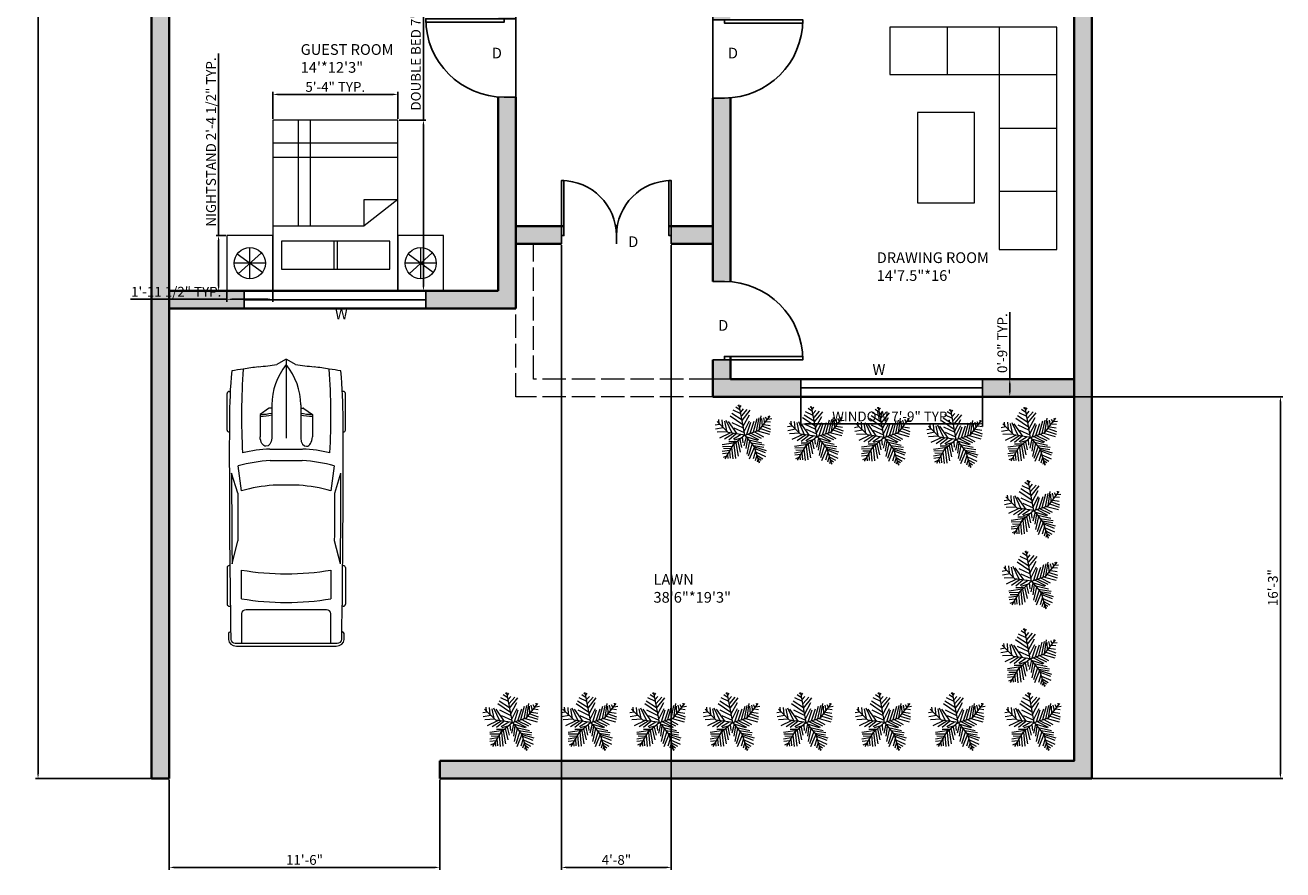
# Model space of a CAD drawing. Units: inches. Extents: x 1658 to 2301, y 1028 to 1972.
# Tile 1 of 2: x 1658 to 2301, y 1028 to 1460. Entities that reach past the tile are written whole.
import ezdxf

# ---------------------------------------------------------------- set-up
doc = ezdxf.new("R2010")
doc.units = ezdxf.units.IN
doc.linetypes.add('ACAD_ISO02W100', pattern=[15, 12, -3])
for name, color, linetype, lineweight in [('A-ANNO-DIMS', 31, 'Continuous', 18), ('A-AREA-IDEN', 31, 'Continuous', 18), ('A-WALL-OVHD', 140, 'ACAD_ISO02W100', 18), ('A-WALL-PATT', 140, 'Continuous', 13), ('DOOR', 54, 'Continuous', 25), ('FUR', 181, 'Continuous', 18), ('L-SITE-VEHI', 8, 'Continuous', 18), ('L-SITE-WALL', 140, 'Continuous', 35), ('TEXT', 31, 'Continuous', 18), ('TREE', 90, 'Continuous', 13), ('WALL', 140, 'Continuous', 35), ('WIND', 211, 'Continuous', 25)]:
    doc.layers.add(name, color=color, linetype=linetype, lineweight=lineweight)
doc.styles.get("Standard").update_dxf_attribs({"font": 'arial.ttf'})
doc.dimstyles.new('ISO-25', dxfattribs={"dimtxt": 5, "dimasz": 2.5, "dimexe": 1.25, "dimexo": 0.625, "dimtad": 1, "dimdec": 0, "dimlunit": 4, "dimtxsty": 'Standard', "dimcen": 2.5, "dimadec": 0, "dimazin": 0, "dimtfac": 1, "dimtdec": 0, "dimtmove": 0, "dimatfit": 3, "dimfxl": 1, "dimarcsym": 0})

# ---------------------------------------------------------------- blocks, each defined once
blk = doc.blocks.new('*U6')
for p, q in [((21.1, 37.41), (21.1, 36.83)), ((46.55, 38.89), (22.35, 38.89)), ((47.8, 37.39), (47.8, 37.41)), ((87.99, 31.87), (74.76, 35.92)), ((134.31, 35.6), (119.29, 31.78)), ((135.45, 37.07), (135.45, 37.41)), ((136.7, 38.89), (160.9, 38.89)), ((162.15, 37.41), (162.15, 36.77)), ((186.47, -33.5), (186.47, 33.5)), ((70.03, 31.54), (86.41, 29.35)), ((138.42, 29.35), (157.25, 29.35)), ((164.52, 26.39), (164.52, -26.39)), ((186.47, 29.35), (167.01, 29.35)), ((188.4, -32.76), (188.4, 32.76)), ((32.27, 11.63), (36.13, 17.17)), ((36.13, 17.17), (50.94, 17.17)), ((29.77, 9.51), (51.68, 9.51)), ((32.12, 9.51), (32.12, 11.15)), ((58.92, -10.77), (58.92, 10.77)), ((66.55, -10.53), (66.55, 10.53)), ((82.74, 8.5), (82.74, -8.5)), ((186.47, -10.53), (186.47, 10.53)), ((3.27, 6.13), (0.1, 0.41)), ((0, 0), (51.68, 0)), ((0.1, -0.41), (3.27, -6.13)), ((29.77, -9.51), (51.68, -9.51)), ((32.12, -9.51), (32.12, -11.15)), ((32.27, -11.63), (36.13, -17.17)), ((36.13, -17.17), (50.94, -17.17)), ((86.41, -29.35), (70.03, -31.54)), ((87.99, -31.87), (74.76, -35.92)), ((134.31, -35.6), (119.29, -31.78)), ((157.25, -29.35), (138.42, -29.35)), ((167.01, -29.35), (186.47, -29.35)), ((21.1, -37.41), (21.1, -36.83)), ((46.55, -38.89), (22.35, -38.89)), ((47.8, -37.39), (47.8, -37.41)), ((135.45, -37.07), (135.45, -37.41)), ((136.7, -38.89), (160.9, -38.89)), ((162.15, -37.41), (162.15, -36.77))]:
    blk.add_line(p, q)
for centre, major_axis, ratio, start_param, end_param in [((266.03, -27.52), (0, 313.31), 0.842304, 1.367076, 1.39176), ((41.19, -490.86), (0, 528.23), 0.842304, 0.00281, 0.075598), ((22.35, 37.41), (0, -1.48), 0.842304, 3.141593, 4.712389), ((64.48, -10555.62), (0, 10593.03), 0.842304, -0.013397, 0.002797), ((46.55, 37.41), (0, 1.48), 0.842304, -1.570796, 0), ((64.48, -10555.62), (0, -10591.55), 0.842304, 3.133765, 3.140441), ((136.7, 37.41), (0, -1.48), 0.842304, 3.141593, 4.712389), ((160.9, 37.41), (0, 1.48), 0.842304, -1.570796, 0), ((180.63, 35.84), (0, 2.22), 0.842304, -0.013017, 1.249894), ((64.48, -10556.36), (0, 10595.31), 0.842304, -0.013397, -0.013017), ((183.98, 33.5), (0, -2.96), 0.842304, 1.570796, 3.128196), ((183.98, 32.76), (0, -5.25), 0.842304, 1.570796, 3.128196), ((259.18, -27.52), (0, -305.3), 0.842304, 4.528606, 4.561838), ((37.47, -593.96), (0, -623.33), 0.842304, 3.096046, 3.200911), ((134.4, 5.39), (0, -89.78), 0.842304, 4.449482, 4.652344), ((135.29, 5.39), (0, 81.77), 0.842304, 1.245306, 1.50788), ((149.6, 2.8), (0, -79.58), 0.842304, 4.372215, 4.640744), ((95.79, -3666.35), (0, -3698.24), 0.842304, 3.134049, 3.144098), ((17.08, 0), (0, 147.02), 0.842304, 4.511394, 4.913384), ((35.91, 0), (0, 147.02), 0.842304, 4.511394, 4.913384), ((167.01, 26.39), (0, 2.96), 0.842304, 0, 1.570796), ((-204.49, 52.4), (0, -250.96), 0.842304, 1.385369, 1.434372), ((13.04, 17.01), (0, 27.42), 0.842304, 4.435146, 4.718221), ((14.2, 17.01), (0, 27.42), 0.842304, 4.435146, 4.718221), ((50.79, 13.34), (6.34, -0.36), 0.603834, -1.395552, 1.581315), ((29.77, -46.66), (0, 56.17), 0.842304, 0, 0.590319), ((32.75, 11.15), (0, 0.74), 0.842304, 0.879714, 1.570796), ((0.62, 0), (0, -0.74), 0.842304, 4.131459, 5.293319), ((-204.49, -52.4), (0, 250.96), 0.842304, -1.434372, -1.385369), ((29.77, 46.66), (0, 56.17), 0.842304, 2.551274, 3.141593), ((32.75, -11.15), (0, -0.74), 0.842304, 4.712389, 5.403472), ((13.04, -17.01), (0, -27.42), 0.842304, 1.564964, 1.848039), ((14.2, -17.01), (0, -27.42), 0.842304, 1.564964, 1.848039), ((134.4, -5.39), (0, -89.78), 0.842304, -1.510751, -1.307889), ((135.29, -5.39), (0, -81.77), 0.842304, -1.50788, -1.245306), ((149.6, -2.8), (0, -79.58), 0.842304, -1.499151, -1.230623), ((259.18, 27.52), (0, 305.3), 0.842304, 1.721348, 1.754579), ((266.03, 27.52), (0, 313.31), 0.842304, 1.749832, 1.774517), ((37.47, 593.96), (0, -623.33), 0.842304, -0.059319, 0.045547), ((95.79, 3666.35), (0, -3698.24), 0.842304, -0.002505, 0.007544), ((167.01, -26.39), (0, -2.96), 0.842304, 4.712389, 6.283185), ((183.98, -32.76), (0, -5.25), 0.842304, 0.013397, 1.570796), ((41.19, 490.86), (0, -528.23), 0.842304, -0.075598, -0.00281), ((22.35, -37.41), (0, 1.48), 0.842304, 1.570796, 3.141593), ((64.48, 10555.62), (0, 10593.03), 0.842304, 3.138796, 3.15499), ((46.55, -37.41), (0, -1.48), 0.842304, 0, 1.570796), ((64.48, 10555.62), (0, -10591.55), 0.842304, 0.001152, 0.007828), ((136.7, -37.41), (0, -1.48), 0.842304, -1.570796, 0), ((160.9, -37.41), (0, 1.48), 0.842304, 3.141593, 4.712389), ((180.63, -35.84), (0, -2.22), 0.842304, -1.249894, 0.013017), ((64.48, 10556.36), (0, 10595.31), 0.842304, 3.15461, 3.15499), ((183.98, -33.5), (0, 2.96), 0.842304, 3.15499, 4.712389)]:
    blk.add_ellipse(centre, major_axis=major_axis, ratio=ratio, start_param=start_param, end_param=end_param)
at = {"extrusion": (0, 0, -1)}
blk.add_ellipse((50.79, -13.34), major_axis=(6.34, 0.36), ratio=0.603834, start_param=-1.395552, end_param=1.581315, dxfattribs=at)
blk = doc.blocks.new('*U2')
for p, q in [((0, 0), (0, -6)), ((40, 0), (40, -6))]:
    blk.add_line(p, q)
blk.add_lwpolyline([(0, 0), (0, 40), (1.75, 40), (1.75, 0)], close=True)
blk.add_arc((0, 0), 40, 0, 90)
blk = doc.blocks.new('*U8')
for p, q in [((-8.737, 47.138), (-17.069, 52.711)), ((-10.186, 53.64), (-13.084, 55.962)), ((0, 0), (-10.5, 57)), ((-9.099, 51.782), (-6.563, 55.962)), ((-7.65, 43.423), (-2.578, 49.46)), ((-5.839, 35.992), (4.667, 48.067)), ((-31.5, 4.5), (-52.5, 25.5)), ((-48.585, 21.131), (-49.309, 29.026)), ((-43.513, 28.561), (-42.427, 15.558)), ((-38.442, 26.239), (-34.819, 7.663)), ((-35.544, 28.097), (-24.314, 3.947)), ((-14.533, 2.09), (-30.834, 25.31)), ((-3.665, 19.273), (-27.574, 35.527)), ((-5.114, 28.097), (-24.676, 40.636)), ((-24.314, 23.917), (-2.941, 13.7)), ((-7.288, 39.707), (-21.778, 46.673)), ((-5.114, 27.632), (10.463, 46.673)), ((-2.941, 16.486), (8.652, 37.85)), ((-1.129, 6.734), (9.014, 26.704)), ((3.942, 1.625), (11.187, 24.381)), ((10.101, 3.483), (17.708, 26.239)), ((16.259, 5.805), (23.142, 31.348)), ((22.055, 7.198), (27.489, 32.277)), ((27, 9), (48, 36)), ((27.127, 9.056), (31.112, 35.992)), ((31.836, 30.883), (32.561, 16.486)), ((35.096, 32.741), (37.27, 22.524)), ((38.719, 34.134), (41.979, 28.561)), ((40.53, 25.775), (48.862, 24.846)), ((43.791, 29.954), (51.036, 30.883)), ((44.153, 36.456), (45.239, 32.741)), ((-47.498, 19.737), (-55.83, 18.344)), ((-40.615, 13.7), (-55.105, 10.913)), ((-33.37, 6.269), (-52.207, 5.34)), ((-28.299, 3.483), (-47.86, -5.805)), ((-21.416, 3.018), (-38.079, -8.128)), ((0, 0), (-31.5, 4.5)), ((-15.982, 2.09), (-30.11, -9.521)), ((0, 0), (-22.5, -19.5)), ((-6.563, 1.161), (-21.416, -8.128)), ((-20.691, 13.7), (-1.129, 4.876)), ((0, 0), (27, 9)), ((0, 0), (18, -22.5)), ((6.478, 1.625), (26.04, -8.592)), ((11.187, 3.483), (30.749, -5.805)), ((18.07, 5.805), (35.096, -3.483)), ((24.229, 7.663), (46.688, 1.625)), ((29.662, 12.307), (48.137, 6.269)), ((33.285, 16.486), (48.862, 10.913)), ((36.183, 19.737), (48.137, 17.88)), ((-17.431, -15.094), (-42.789, -18.809)), ((-24.314, -21.596), (-42.427, -22.06)), ((-22.5, -19.5), (-37.5, -45)), ((-15.257, -12.772), (-30.11, -12.772)), ((-20.691, -18.345), (-17.793, -44.352)), ((-6.563, -5.805), (-19.967, -9.985)), ((-17.069, -15.094), (-12.721, -40.172)), ((-13.446, -11.378), (-8.737, -32.741)), ((-9.461, -8.592), (-6.201, -23.453)), ((-4.752, -3.483), (-3.665, -14.629)), ((2.493, -3.019), (-1.491, -20.202)), ((1.769, -2.555), (24.229, -9.521)), ((5.029, -6.27), (2.131, -25.775)), ((9.014, -11.378), (3.58, -35.992)), ((14.085, -16.951), (6.478, -40.172)), ((7.565, -9.056), (32.198, -14.629)), ((18.07, -22.524), (8.289, -45.745)), ((12.274, -15.094), (36.907, -18.809)), ((16.259, -19.738), (36.183, -22.989)), ((18, -22.5), (27, -52.5)), ((18.433, -22.524), (40.53, -29.026)), ((-28.299, -29.026), (-42.789, -31.348)), ((-30.834, -34.135), (-42.427, -35.528)), ((-34.457, -39.708), (-40.978, -42.494)), ((-26.849, -26.24), (-40.253, -25.775)), ((-32.646, -36.921), (-31.921, -44.352)), ((-29.023, -30.884), (-27.936, -43.887)), ((-25.038, -23.918), (-22.865, -45.281)), ((20.244, -30.419), (15.897, -44.816)), ((19.157, -25.311), (38.719, -33.206)), ((22.78, -37.85), (19.519, -48.532)), ((21.331, -32.741), (39.081, -40.636)), ((22.78, -38.314), (34.372, -44.816)), ((24.591, -45.745), (23.142, -50.854)), ((24.591, -43.423), (30.749, -47.603)), ((26.764, -49.925), (28.213, -50.854))]:
    blk.add_line(p, q)
blk = doc.blocks.new('*D10')
at = {"layer": 'A-ANNO-DIMS', "color": 0, "lineweight": -2, "transparency": 16777216}
for p, q in [((1722.37, 1915.04), (1663.75, 1915.04)), ((1665, 1912.54), (1665, 1077.54)), ((1722.37, 1075.04), (1663.75, 1075.04))]:
    blk.add_line(p, q, dxfattribs=at)
at = {"layer": 'A-ANNO-DIMS', "color": 0, "lineweight": 100, "transparency": 16777216}
for points in [[(1664.59, 1912.54), (1665.42, 1912.54), (1665, 1915.04)], [(1664.59, 1077.54), (1665.42, 1077.54), (1665, 1075.04)]]:
    blk.add_solid(points, dxfattribs=at)
at = {"layer": 'Defpoints', "color": 0, "lineweight": 100, "transparency": 16777216}
for p in [(1722.99, 1915.04), (1665, 1075.04), (1722.99, 1075.04)]:
    blk.add_point(p, dxfattribs=at)
at = {"layer": 'A-ANNO-DIMS', "color": 0, "transparency": 16777216, "insert": (1661.82, 1495.04), "char_height": 5, "attachment_point": 5, "rotation": 90}
blk.add_mtext("70'", dxfattribs=at)
blk = doc.blocks.new('BED-DOUBLE')
for p, q in [((33.2, 63.87), (33.2, 17.24)), ((68.25, 63.87), (68.25, 0)), ((75.56, 63.87), (75.56, 0)), ((33.2, 50.75), (87.28, 50.75)), ((33.2, 44.52), (87.28, 44.52)), ((33.2, 17.24), (46.75, 17.24)), ((46.75, 0), (33.2, 17.24)), ((46.75, 17.24), (46.75, 0))]:
    blk.add_line(p, q)
for points in [[(0, 0), (87.28, 0), (87.28, 63.87), (0, 63.87)], [(11.05, 30.77), (25.46, 30.77), (25.46, 59.34), (11.05, 59.34)], [(11.05, 4.13), (25.46, 4.13), (25.46, 32.7), (11.05, 32.7)]]:
    blk.add_lwpolyline(points, close=True)
blk = doc.blocks.new('NIGHTSTAND-LAMP')
for p, q in [((14.17, 3.75), (14.17, 19.65)), ((19.52, 5.82), (8.81, 17.58)), ((9.46, 5.29), (18.87, 18.1)), ((6.22, 11.7), (22.11, 11.7))]:
    blk.add_line(p, q)
blk.add_lwpolyline([(0, 0), (28.33, 0), (28.33, 23.39), (0, 23.39)], close=True)
blk.add_circle((14.17, 11.7), 7.95)
blk = doc.blocks.new('WIN-93')
blk.add_line((0, 4.5), (92.82, 4.5))
blk.add_lwpolyline([(0, 0), (92.82, 0), (92.82, 9), (0, 9)], close=True)
blk = doc.blocks.new('*D17')
at = {"layer": 'A-ANNO-DIMS', "color": 0, "lineweight": -2, "transparency": 16777216}
for p, q in [((1861.79, 1411.32), (1861.79, 1503.92)), ((1849.32, 1411.32), (1863.04, 1411.32)), ((1861.79, 1326.54), (1861.79, 1408.82)), ((1849.32, 1324.04), (1863.04, 1324.04))]:
    blk.add_line(p, q, dxfattribs=at)
at = {"layer": 'A-ANNO-DIMS', "color": 0, "lineweight": 100, "transparency": 16777216}
for points in [[(1861.37, 1408.82), (1862.2, 1408.82), (1861.79, 1411.32)], [(1861.37, 1326.54), (1862.2, 1326.54), (1861.79, 1324.04)]]:
    blk.add_solid(points, dxfattribs=at)
at = {"layer": 'Defpoints', "color": 0, "lineweight": 100, "transparency": 16777216}
for p in [(1848.69, 1411.32), (1861.79, 1411.32), (1848.69, 1324.04)]:
    blk.add_point(p, dxfattribs=at)
at = {"layer": 'A-ANNO-DIMS', "color": 0, "transparency": 16777216, "insert": (1858.57, 1458.87), "char_height": 5, "attachment_point": 5, "rotation": 90}
blk.add_mtext('DOUBLE BED 7\'-3 1/2" TYP.', dxfattribs=at)
blk = doc.blocks.new('*D18')
at = {"layer": 'A-ANNO-DIMS', "color": 0, "lineweight": -2, "transparency": 16777216}
for p, q in [((1784.83, 1411.94), (1784.83, 1425.66)), ((1848.69, 1411.94), (1848.69, 1425.66)), ((1846.19, 1424.41), (1787.33, 1424.41))]:
    blk.add_line(p, q, dxfattribs=at)
at = {"layer": 'A-ANNO-DIMS', "color": 0, "lineweight": 100, "transparency": 16777216}
for points in [[(1787.33, 1424.83), (1787.33, 1423.99), (1784.83, 1424.41)], [(1846.19, 1424.83), (1846.19, 1423.99), (1848.69, 1424.41)]]:
    blk.add_solid(points, dxfattribs=at)
at = {"layer": 'Defpoints', "color": 0, "lineweight": 100, "transparency": 16777216}
for p in [(1784.83, 1424.41), (1784.83, 1411.32), (1848.69, 1411.32)]:
    blk.add_point(p, dxfattribs=at)
at = {"layer": 'A-ANNO-DIMS', "color": 0, "transparency": 16777216, "insert": (1816.76, 1427.58), "char_height": 5, "attachment_point": 5}
blk.add_mtext('5\'-4" TYP.', dxfattribs=at)
blk = doc.blocks.new('*D19')
at = {"layer": 'A-ANNO-DIMS', "color": 0, "lineweight": -2, "transparency": 16777216}
for p, q in [((1757.19, 1352.37), (1757.19, 1445.35)), ((1760.81, 1352.37), (1755.94, 1352.37)), ((1757.19, 1326.54), (1757.19, 1349.87)), ((1760.81, 1324.04), (1755.94, 1324.04))]:
    blk.add_line(p, q, dxfattribs=at)
at = {"layer": 'A-ANNO-DIMS', "color": 0, "lineweight": 100, "transparency": 16777216}
for points in [[(1756.77, 1349.87), (1757.6, 1349.87), (1757.19, 1352.37)], [(1756.77, 1326.54), (1757.6, 1326.54), (1757.19, 1324.04)]]:
    blk.add_solid(points, dxfattribs=at)
at = {"layer": 'Defpoints', "color": 0, "lineweight": 100, "transparency": 16777216}
for p in [(1757.19, 1352.37), (1761.43, 1352.37), (1761.43, 1324.04)]:
    blk.add_point(p, dxfattribs=at)
at = {"layer": 'A-ANNO-DIMS', "color": 0, "transparency": 16777216, "insert": (1753.97, 1400.11), "char_height": 5, "attachment_point": 5, "rotation": 90}
blk.add_mtext('NIGHTSTAND 2\'-4 1/2" TYP.', dxfattribs=at)
blk = doc.blocks.new('*D20')
at = {"layer": 'A-ANNO-DIMS', "color": 0, "lineweight": -2, "transparency": 16777216}
for p, q in [((1761.43, 1323.41), (1761.43, 1318.54)), ((1784.83, 1323.41), (1784.83, 1318.54)), ((1761.43, 1319.79), (1712.14, 1319.79)), ((1782.33, 1319.79), (1763.93, 1319.79))]:
    blk.add_line(p, q, dxfattribs=at)
at = {"layer": 'A-ANNO-DIMS', "color": 0, "lineweight": 100, "transparency": 16777216}
for points in [[(1763.93, 1320.21), (1763.93, 1319.37), (1761.43, 1319.79)], [(1782.33, 1320.21), (1782.33, 1319.37), (1784.83, 1319.79)]]:
    blk.add_solid(points, dxfattribs=at)
at = {"layer": 'Defpoints', "color": 0, "lineweight": 100, "transparency": 16777216}
for p in [(1761.43, 1324.04), (1784.83, 1324.04), (1761.43, 1319.79)]:
    blk.add_point(p, dxfattribs=at)
at = {"layer": 'A-ANNO-DIMS', "color": 0, "transparency": 16777216, "insert": (1735.54, 1323), "char_height": 5, "attachment_point": 5}
blk.add_mtext('1\'-11 1/2" TYP.', dxfattribs=at)
blk = doc.blocks.new('*D23')
at = {"layer": 'A-ANNO-DIMS', "color": 0, "lineweight": -2, "transparency": 16777216}
for p, q in [((2054.42, 1269.41), (2054.42, 1254.86)), ((2147.24, 1269.41), (2147.24, 1254.86)), ((2056.92, 1256.11), (2144.74, 1256.11))]:
    blk.add_line(p, q, dxfattribs=at)
at = {"layer": 'A-ANNO-DIMS', "color": 0, "lineweight": 100, "transparency": 16777216}
for points in [[(2056.92, 1256.53), (2056.92, 1255.7), (2054.42, 1256.11)], [(2144.74, 1256.53), (2144.74, 1255.7), (2147.24, 1256.11)]]:
    blk.add_solid(points, dxfattribs=at)
at = {"layer": 'Defpoints', "color": 0, "lineweight": 100, "transparency": 16777216}
for p in [(2054.42, 1270.04), (2147.24, 1270.04), (2147.24, 1256.11)]:
    blk.add_point(p, dxfattribs=at)
at = {"layer": 'A-ANNO-DIMS', "color": 0, "transparency": 16777216, "insert": (2100.83, 1259.33), "char_height": 5, "attachment_point": 5}
blk.add_mtext('WINDOW 7\'-9" TYP.', dxfattribs=at)
blk = doc.blocks.new('*D24')
at = {"layer": 'A-ANNO-DIMS', "color": 0, "lineweight": -2, "transparency": 16777216}
for p, q in [((2161.17, 1279.04), (2161.17, 1313.27)), ((2147.87, 1279.04), (2162.42, 1279.04)), ((2161.17, 1272.54), (2161.17, 1276.54)), ((2147.87, 1270.04), (2162.42, 1270.04))]:
    blk.add_line(p, q, dxfattribs=at)
at = {"layer": 'A-ANNO-DIMS', "color": 0, "lineweight": 100, "transparency": 16777216}
for points in [[(2160.75, 1276.54), (2161.58, 1276.54), (2161.17, 1279.04)], [(2160.75, 1272.54), (2161.58, 1272.54), (2161.17, 1270.04)]]:
    blk.add_solid(points, dxfattribs=at)
at = {"layer": 'Defpoints', "color": 0, "lineweight": 100, "transparency": 16777216}
for p in [(2147.24, 1279.04), (2161.17, 1279.04), (2147.24, 1270.04)]:
    blk.add_point(p, dxfattribs=at)
at = {"layer": 'A-ANNO-DIMS', "color": 0, "transparency": 16777216, "insert": (2157.99, 1297.4), "char_height": 5, "attachment_point": 5, "rotation": 90}
blk.add_mtext('0\'-9" TYP.', dxfattribs=at)
blk = doc.blocks.new('*D29')
at = {"layer": 'A-ANNO-DIMS', "color": 0, "lineweight": -2, "transparency": 16777216}
for p, q in [((2194.62, 1270.04), (2300.59, 1270.04)), ((2299.34, 1267.54), (2299.34, 1077.54)), ((2203.62, 1075.04), (2300.59, 1075.04))]:
    blk.add_line(p, q, dxfattribs=at)
at = {"layer": 'A-ANNO-DIMS', "color": 0, "lineweight": 100, "transparency": 16777216}
for points in [[(2298.92, 1267.54), (2299.76, 1267.54), (2299.34, 1270.04)], [(2298.92, 1077.54), (2299.76, 1077.54), (2299.34, 1075.04)]]:
    blk.add_solid(points, dxfattribs=at)
at = {"layer": 'Defpoints', "color": 0, "lineweight": 100, "transparency": 16777216}
for p in [(2193.99, 1270.04), (2202.99, 1075.04), (2299.34, 1075.04)]:
    blk.add_point(p, dxfattribs=at)
at = {"layer": 'A-ANNO-DIMS', "color": 0, "transparency": 16777216, "insert": (2296.16, 1172.54), "char_height": 5, "attachment_point": 5, "rotation": 90}
blk.add_mtext('16\'-3"', dxfattribs=at)
blk = doc.blocks.new('*D30')
at = {"layer": 'A-ANNO-DIMS', "color": 0, "lineweight": -2, "transparency": 16777216}
for p, q in [((1731.99, 1074.41), (1731.99, 1028.44)), ((1870.11, 1074.41), (1870.11, 1028.44)), ((1734.49, 1029.69), (1867.61, 1029.69))]:
    blk.add_line(p, q, dxfattribs=at)
at = {"layer": 'A-ANNO-DIMS', "color": 0, "lineweight": 100, "transparency": 16777216}
for points in [[(1734.49, 1030.1), (1734.49, 1029.27), (1731.99, 1029.69)], [(1867.61, 1030.1), (1867.61, 1029.27), (1870.11, 1029.69)]]:
    blk.add_solid(points, dxfattribs=at)
at = {"layer": 'Defpoints', "color": 0, "lineweight": 100, "transparency": 16777216}
for p in [(1731.99, 1075.04), (1870.11, 1075.04), (1870.11, 1029.69)]:
    blk.add_point(p, dxfattribs=at)
at = {"layer": 'A-ANNO-DIMS', "color": 0, "transparency": 16777216, "insert": (1801.05, 1032.87), "char_height": 5, "attachment_point": 5}
blk.add_mtext('11\'-6"', dxfattribs=at)
blk = doc.blocks.new('*D31')
at = {"layer": 'A-ANNO-DIMS', "color": 0, "lineweight": -2, "transparency": 16777216}
for p, q in [((1908.99, 1357.76), (1908.99, 1961.64)), ((1911.49, 1960.39), (2006.99, 1960.39)), ((2009.49, 1357.76), (2009.49, 1961.64))]:
    blk.add_line(p, q, dxfattribs=at)
at = {"layer": 'A-ANNO-DIMS', "color": 0, "lineweight": 100, "transparency": 16777216}
for points in [[(1911.49, 1960.8), (1911.49, 1959.97), (1908.99, 1960.39)], [(2006.99, 1960.8), (2006.99, 1959.97), (2009.49, 1960.39)]]:
    blk.add_solid(points, dxfattribs=at)
at = {"layer": 'Defpoints', "color": 0, "lineweight": 100, "transparency": 16777216}
for p in [(2009.49, 1960.39), (1908.99, 1357.13), (2009.49, 1357.13)]:
    blk.add_point(p, dxfattribs=at)
at = {"layer": 'A-ANNO-DIMS', "color": 0, "transparency": 16777216, "insert": (1959.24, 1963.6), "char_height": 5, "attachment_point": 5}
blk.add_mtext('8\'-4 1/2"', dxfattribs=at)
blk = doc.blocks.new('*D32')
at = {"layer": 'A-ANNO-DIMS', "color": 0, "lineweight": -2, "transparency": 16777216}
for p, q in [((1932.24, 1347.51), (1932.24, 1028.44)), ((1988.35, 1347.51), (1988.35, 1028.44)), ((1934.74, 1029.69), (1985.85, 1029.69))]:
    blk.add_line(p, q, dxfattribs=at)
at = {"layer": 'A-ANNO-DIMS', "color": 0, "lineweight": 100, "transparency": 16777216}
for points in [[(1934.74, 1030.1), (1934.74, 1029.27), (1932.24, 1029.69)], [(1985.85, 1030.1), (1985.85, 1029.27), (1988.35, 1029.69)]]:
    blk.add_solid(points, dxfattribs=at)
at = {"layer": 'Defpoints', "color": 0, "lineweight": 100, "transparency": 16777216}
for p in [(1932.24, 1348.13), (1988.35, 1348.13), (1988.35, 1029.69)]:
    blk.add_point(p, dxfattribs=at)
at = {"layer": 'A-ANNO-DIMS', "color": 0, "transparency": 16777216, "insert": (1960.3, 1032.87), "char_height": 5, "attachment_point": 5}
blk.add_mtext('4\'-8"', dxfattribs=at)

msp = doc.modelspace()

# ---------------------------------------------------------------- hatches: boundary and pattern name
at = {"layer": 'A-WALL-PATT'}
h = msp.add_hatch(color=256, dxfattribs=at)
h.dxf.hatch_style = 1
h.paths.add_polyline_path([(1731.99, 1315.04), (1731.99, 1906.04), (2193.99, 1906.04), (2193.99, 1084.04), (1870.11, 1084.04), (1870.11, 1075.04), (2202.99, 1075.04), (2202.99, 1915.04), (1722.99, 1915.04), (1722.99, 1075.04), (1731.99, 1075.04), (1731.99, 1084.04)])
h = msp.add_hatch(color=256, dxfattribs=at)
h.dxf.hatch_style = 1
h.paths.add_polyline_path([(1779.42, 1699.04), (1731.99, 1699.04), (1731.99, 1697.54), (1731.99, 1694.54), (1779.42, 1694.54)])
h.paths.add_polyline_path([(1816.49, 1672.04), (1811.99, 1672.04), (1811.99, 1640.54), (1811.99, 1480.04), (1816.49, 1480.04)])
h.paths.add_polyline_path([(1811.99, 1610.54), (1731.99, 1610.54), (1731.99, 1606.04), (1811.99, 1606.04)])
h.paths.add_polyline_path([(1811.99, 1568.54), (1731.99, 1568.54), (1731.99, 1564.04), (1811.99, 1564.04)])
h.paths.add_polyline_path([(1738.02, 1480.04), (1731.99, 1480.04), (1731.99, 1471.04), (1738.02, 1471.04), (1738.02, 1475.43)])
h.paths.add_polyline_path([(1908.99, 1480.04), (1766.9, 1480.04, -0.039614), (1767.27, 1475.43), (1767.27, 1471.04), (1899.99, 1471.04), (1899.99, 1463.03), (1902.99, 1463.03), (1908.99, 1463.03)])
h.paths.add_polyline_path([(1908.99, 1423.03), (1902.99, 1423.03, -0.01877), (1899.99, 1423.14), (1899.99, 1324.04), (1863.03, 1324.04), (1863.03, 1315.04), (1908.99, 1315.04)])
h.paths.add_polyline_path([(1770.21, 1324.04), (1761.43, 1324.04), (1731.99, 1324.04), (1731.99, 1315.04), (1770.21, 1315.04)])
h.paths.add_polyline_path([(2009.49, 1357.13), (1988.35, 1357.13), (1988.35, 1352.34), (1988.35, 1348.13), (2009.49, 1348.13)])
h.paths.add_polyline_path([(1932.24, 1352.34), (1932.24, 1357.13), (1908.99, 1357.13), (1908.99, 1348.13), (1932.24, 1348.13)])
h.paths.add_polyline_path([(2018.49, 1422.69, -0.01877), (2015.49, 1422.57), (2009.49, 1422.57), (2009.49, 1328.83), (2015.49, 1328.83, -0.01877), (2018.49, 1328.71)])
h.paths.add_polyline_path([(2054.42, 1279.04), (2018.49, 1279.04), (2009.49, 1279.04), (2009.49, 1270.04), (2054.42, 1270.04)])
h.paths.add_polyline_path([(2018.49, 1288.83), (2015.49, 1288.83), (2009.49, 1288.83), (2009.49, 1279.04), (2018.49, 1279.04)])
h.paths.add_polyline_path([(2193.99, 1279.04), (2147.24, 1279.04), (2147.24, 1270.04), (2193.99, 1270.04)])
h.paths.add_polyline_path([(2061.99, 1480.04), (2009.49, 1480.04), (2009.49, 1462.57), (2015.49, 1462.57), (2018.49, 1462.57), (2018.49, 1471.04), (2061.99, 1471.04)])
h.paths.add_polyline_path([(2193.99, 1480.04), (2169.99, 1480.04), (2066.49, 1480.04), (2066.49, 1522.24), (2061.99, 1522.24), (2061.99, 1471.04), (2193.99, 1471.04)])
h.paths.add_polyline_path([(2066.49, 1600.04), (2061.99, 1600.04), (2061.99, 1572.51), (2066.49, 1572.51)])
h.paths.add_polyline_path([(2066.49, 1672.04), (2061.99, 1672.04), (2061.99, 1657.22), (2066.49, 1657.22)])
h.paths.add_polyline_path([(2132.49, 1604.54), (2127.99, 1604.54), (2066.49, 1604.54), (2066.49, 1620.73), (2061.99, 1620.73), (2061.99, 1600.04), (2132.49, 1600.04)])
h.paths.add_polyline_path([(2132.49, 1672.04), (2127.99, 1672.04), (2127.99, 1604.54), (2132.49, 1604.54)])
h.paths.add_polyline_path([(2193.99, 1604.54), (2166.96, 1604.54), (2166.96, 1600.04), (2193.99, 1600.04)])
h.paths.add_polyline_path([(2193.99, 1681.04), (2014.55, 1681.04, -0.01877), (2014.67, 1678.04), (2014.67, 1672.04), (2193.99, 1672.04)])
h.paths.add_polyline_path([(2166.4, 1681.92), (2166.4, 1747.55), (2145.97, 1747.55), (2145.97, 1681.92)], flags=9)
h.paths.add_polyline_path([(1915.65, 1653.85), (1929.01, 1653.85), (1929.01, 1665.13), (1915.65, 1665.13)], flags=9)
h.paths.add_polyline_path([(2138.45, 1814.92), (2185.37, 1814.92), (2185.37, 1835.35), (2138.45, 1835.35)], flags=9)
h.paths.add_polyline_path([(1981.17, 1881.08), (2028.95, 1881.08), (2028.95, 1901.5), (1981.17, 1901.5)], flags=9)
h.paths.add_polyline_path([(1867.78, 1703.2), (1910.3, 1703.2), (1910.3, 1723.63), (1867.78, 1723.63)], flags=9)
h.paths.add_polyline_path([(2031.55, 1705.85), (2074.07, 1705.85), (2074.07, 1726.27), (2031.55, 1726.27)], flags=9)
h.paths.add_polyline_path([(1943.61, 1572), (2023.69, 1572), (2023.69, 1592.42), (1943.61, 1592.42)], flags=9)
h.paths.add_polyline_path([(2071.73, 1627.4), (2128.87, 1627.4), (2128.87, 1647.83), (2071.73, 1647.83)], flags=9)
h.paths.add_polyline_path([(2143.67, 1623.1), (2195.26, 1623.1), (2195.26, 1643.52), (2143.67, 1643.52)], flags=9)
h.paths.add_polyline_path([(2101.19, 1540.97), (2137.76, 1540.97), (2137.76, 1561.39), (2101.19, 1561.39)], flags=9)
h.paths.add_polyline_path([(2091.03, 1326.07), (2156.87, 1326.07), (2156.87, 1346.5), (2091.03, 1346.5)], flags=9)
h.paths.add_polyline_path([(1796.89, 1432.36), (1852.31, 1432.36), (1852.31, 1452.79), (1796.89, 1452.79)], flags=9)
h.paths.add_polyline_path([(1751.02, 1530.9), (1797.94, 1530.9), (1797.94, 1551.32), (1751.02, 1551.32)], flags=9)
h.paths.add_polyline_path([(1747.18, 1642.43), (1802.17, 1642.43), (1802.17, 1662.86), (1747.18, 1662.86)], flags=9)
h.paths.add_polyline_path([(1805.32, 1731.07), (1805.32, 1796.71), (1784.9, 1796.71), (1784.9, 1731.07)], flags=9)
h.paths.add_polyline_path([(1741.72, 1875.52), (1788.64, 1875.52), (1788.64, 1895.95), (1741.72, 1895.95)], flags=9)

# ---------------------------------------------------------------- linework, layer by layer
at = {"layer": 'A-WALL-OVHD'}
for p, q in [((1918.01, 1279.04), (1918.01, 1348.13)), ((1908.99, 1270.04), (1908.99, 1315.04)), ((2009.49, 1279.04), (1918.01, 1279.04)), ((2018.49, 1279.04), (2009.49, 1279.04)), ((2009.49, 1270.04), (1908.99, 1270.04))]:
    msp.add_line(p, q, dxfattribs=at)
at = {"layer": 'FUR'}
for p, q in [((2129.24, 1458.73), (2129.24, 1434.55)), ((2155.71, 1407.14), (2185.21, 1407.14)), ((2155.71, 1374.96), (2185.21, 1374.96))]:
    msp.add_line(p, q, dxfattribs=at)
for points in [[(2185.21, 1458.73), (2099.88, 1458.73), (2099.88, 1434.55), (2185.21, 1434.55)], [(2185.21, 1458.73), (2155.71, 1458.73), (2155.71, 1345.19), (2185.21, 1345.19)], [(2143.07, 1415.18), (2114.13, 1415.18), (2114.13, 1369.04), (2143.07, 1369.04)]]:
    msp.add_lwpolyline(points, close=True, dxfattribs=at)
at = {"layer": 'L-SITE-WALL'}
for p, q in [((1722.99, 1075.04), (1722.99, 1915.04)), ((2202.99, 1915.04), (2202.99, 1075.04)), ((1731.99, 1084.04), (1731.99, 1315.04)), ((1731.99, 1084.04), (1731.99, 1075.04)), ((1870.11, 1084.04), (1870.11, 1075.04)), ((1731.99, 1075.04), (1722.99, 1075.04)), ((2202.99, 1075.04), (1870.11, 1075.04))]:
    msp.add_line(p, q, dxfattribs=at)
for points in [[(1731.99, 1075.04), (1722.99, 1075.04), (1722.99, 1915.04), (2202.99, 1915.04), (2202.99, 1075.04), (1870.11, 1075.04)], [(1731.99, 1084.04), (1731.99, 1906.04), (2193.99, 1906.04), (2193.99, 1084.04), (1870.11, 1084.04)]]:
    msp.add_lwpolyline(points, dxfattribs=at)
at = {"layer": 'WALL'}
for p, q in [((2193.99, 1471.04), (2193.99, 1279.04)), ((1899.99, 1324.04), (1899.99, 1423.14)), ((1899.99, 1324.04), (1899.99, 1423.14)), ((1908.99, 1315.04), (1908.99, 1423.03)), ((2009.49, 1328.83), (2009.49, 1422.57)), ((2018.49, 1328.71), (2018.49, 1422.69)), ((1908.99, 1357.13), (1933.47, 1357.13)), ((1959.88, 1357.13), (1960.71, 1357.13)), ((1987.12, 1357.13), (2009.49, 1357.13)), ((1908.99, 1348.13), (1932.24, 1348.13)), ((1988.35, 1348.13), (2009.49, 1348.13)), ((1731.99, 1324.04), (1899.99, 1324.04)), ((1731.99, 1324.04), (1899.99, 1324.04)), ((1731.99, 1315.04), (1908.99, 1315.04)), ((1731.99, 1315.04), (1908.99, 1315.04)), ((1899.99, 1315.04), (1908.99, 1315.04)), ((2009.49, 1270.04), (2009.49, 1288.83)), ((2018.49, 1279.04), (2018.49, 1290.58)), ((2193.99, 1279.04), (2018.49, 1279.04)), ((2193.99, 1270.04), (2009.49, 1270.04))]:
    msp.add_line(p, q, dxfattribs=at)

# ---------------------------------------------------------------- block references
at = {"layer": 'DOOR', "xscale": -1}
for p, rotation in [((1902.99, 1463.03), 90), ((2015.49, 1288.83), 270)]:
    msp.add_blockref('*U2', p, dxfattribs=dict(at, rotation=rotation))
at = {"layer": 'DOOR', "rotation": 270}
msp.add_blockref('*U2', (2015.49, 1462.57), dxfattribs=at)
at = {"layer": 'DOOR', "yscale": 0.7012744155392432, "zscale": 0.7012744155392432}
for p, xscale in [((1932.24, 1352.34), 0.7012744155392432), ((1988.35, 1352.34), -0.7012744155392432)]:
    msp.add_blockref('*U2', p, dxfattribs=dict(at, xscale=xscale))
at = {"layer": 'FUR'}
for name, p, rotation in [('BED-DOUBLE', (1848.69, 1324.04), 89.9999999999992), ('NIGHTSTAND-LAMP', (1784.83, 1324.04), 90.00000000000222), ('NIGHTSTAND-LAMP', (1872.09, 1324.04), 90.0000000000017)]:
    msp.add_blockref(name, p, dxfattribs=dict(at, rotation=rotation))
at = {"layer": 'L-SITE-VEHI', "xscale": 0.7771995421733044, "yscale": 0.7771995421733044, "zscale": 0.7771995421733044, "rotation": 270}
msp.add_blockref('*U6', (1791.74, 1289.11), dxfattribs=at)
at = {"layer": 'TREE', "xscale": 0.2701622865199739, "yscale": 0.2701622865199739, "zscale": 0.2701622865199739}
for p in [(2025.86, 1250.49), (2062.81, 1249.72), (2096.98, 1249.28), (2133.82, 1248.16), (2171.78, 1249.28), (2173.39, 1211.95), (2172.32, 1175.9), (2171.53, 1136.25), (1907.17, 1103.62), (1947.19, 1103.62), (1982.23, 1103.62), (2019.73, 1103.62), (2057.23, 1103.62), (2097.25, 1103.62), (2134.75, 1103.62), (2173.69, 1103.62)]:
    msp.add_blockref('*U8', p, dxfattribs=at)
at = {"layer": 'WIND'}
for p in [(1770.21, 1315.04), (2054.42, 1270.04)]:
    msp.add_blockref('WIN-93', p, dxfattribs=at)

# ---------------------------------------------------------------- texts
at = {"layer": 'A-AREA-IDEN', "attachment_point": 1}
for s, insert, char_height in [('GUEST ROOM\\P14\'*12\'3"', (1799.1, 1450.07), 5.473), ('DRAWING ROOM\\P14\'7.5"*16\'', (2093.23, 1343.78), 5.4735), ('LAWN\\P38\'6"*19\'3"', (1979.24, 1179.46), 5.4735)]:
    msp.add_mtext_dynamic_manual_height_columns(s, width=109.1079, gutter_width=27.37, heights=[0], dxfattribs=dict(at, insert=insert, char_height=char_height))
at = {"layer": 'TEXT', "char_height": 5.47, "attachment_point": 1}
for s, insert in [('D', (1896.71, 1448.25)), ('D', (2017.25, 1448.25)), ('D', (1966.36, 1351.93)), ('W', (1816.6, 1315.04)), ('D', (2012.29, 1309.2)), ('W', (2091.07, 1286.67))]:
    msp.add_mtext_dynamic_manual_height_columns(s, width=109.1079, gutter_width=27.37, heights=[0], dxfattribs=dict(at, insert=insert))

# ---------------------------------------------------------------- dimensions: what is measured, and where the dimension line sits
at = {"layer": 'A-ANNO-DIMS'}
for base, p1, p2, picture, middle in [((2009.49, 1960.39), (1908.99, 1357.13), (2009.49, 1357.13), '*D31', (1959.24, 1963.6)), ((1988.35, 1029.69), (1932.24, 1348.13), (1988.35, 1348.13), '*D32', (1960.3, 1032.87)), ((1870.11, 1029.69), (1731.99, 1075.04), (1870.11, 1075.04), '*D30', (1801.05, 1032.87))]:
    dim = msp.add_linear_dim(base=base, p1=p1, p2=p2, dimstyle='ISO-25', override={"dimdec": 1, "dimlfac": 1, "dimrnd": 0, "dimzin": 1, "dimdsep": 46, "dimlunit": 4, "dimfrac": 2}, dxfattribs=at)
    dim.commit()
    dim.dimension.update_dxf_attribs({"geometry": picture, "text_midpoint": middle})
for base, p1, p2, override, picture, middle in [((1665, 1075.04), (1722.99, 1915.04), (1722.99, 1075.04), {"dimclrd": 0, "dimclre": 0, "dimclrt": 0}, '*D10', (1661.82, 1495.04)), ((2299.34, 1075.04), (2193.99, 1270.04), (2202.99, 1075.04), {"dimdec": 1, "dimlfac": 1, "dimrnd": 0, "dimzin": 1, "dimdsep": 46, "dimlunit": 4, "dimfrac": 2}, '*D29', (2296.16, 1172.54))]:
    dim = msp.add_linear_dim(base=base, p1=p1, p2=p2, angle=90, dimstyle='ISO-25', override=override, dxfattribs=at)
    dim.commit()
    dim.dimension.update_dxf_attribs({"geometry": picture, "text_midpoint": middle})
for base, p1, p2, angle, text, picture, middle in [((1861.79, 1411.32), (1848.69, 1324.04), (1848.69, 1411.32), 90, 'DOUBLE BED <> TYP.', '*D17', (1858.57, 1458.87)), ((1757.19, 1352.37), (1761.43, 1324.04), (1761.43, 1352.37), 90, 'NIGHTSTAND <> TYP.', '*D19', (1753.97, 1400.11)), ((1784.83, 1424.41), (1848.69, 1411.32), (1784.83, 1411.32), 180, '<> TYP.', '*D18', (1816.76, 1427.58)), ((1761.43, 1319.79), (1784.83, 1324.04), (1761.43, 1324.04), 180, '<> TYP.', '*D20', (1735.54, 1323)), ((2161.17, 1279.04), (2147.24, 1270.04), (2147.24, 1279.04), 90, '<> TYP.', '*D24', (2157.99, 1297.4))]:
    dim = msp.add_linear_dim(base=base, p1=p1, p2=p2, angle=angle, text=text, dimstyle='ISO-25', override={"dimdec": 1, "dimlfac": 1, "dimrnd": 0, "dimzin": 1, "dimdsep": 46, "dimlunit": 4, "dimfrac": 2}, dxfattribs=at)
    dim.commit()
    dim.dimension.update_dxf_attribs({"geometry": picture, "text_midpoint": middle})
dim = msp.add_linear_dim(base=(2147.24, 1256.11), p1=(2054.42, 1270.04), p2=(2147.24, 1270.04), text='WINDOW <> TYP.', dimstyle='ISO-25', override={"dimdec": 1, "dimlfac": 1, "dimrnd": 0, "dimzin": 1, "dimdsep": 46, "dimlunit": 4, "dimfrac": 2}, dxfattribs=at)
dim.commit()
dim.dimension.update_dxf_attribs({"geometry": '*D23', "text_midpoint": (2100.83, 1259.33)})

doc.saveas('drawing.dxf')
